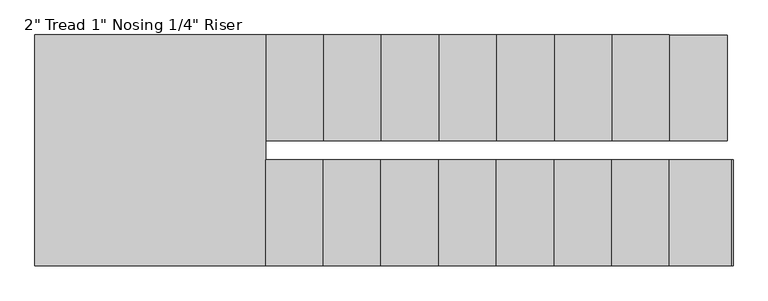
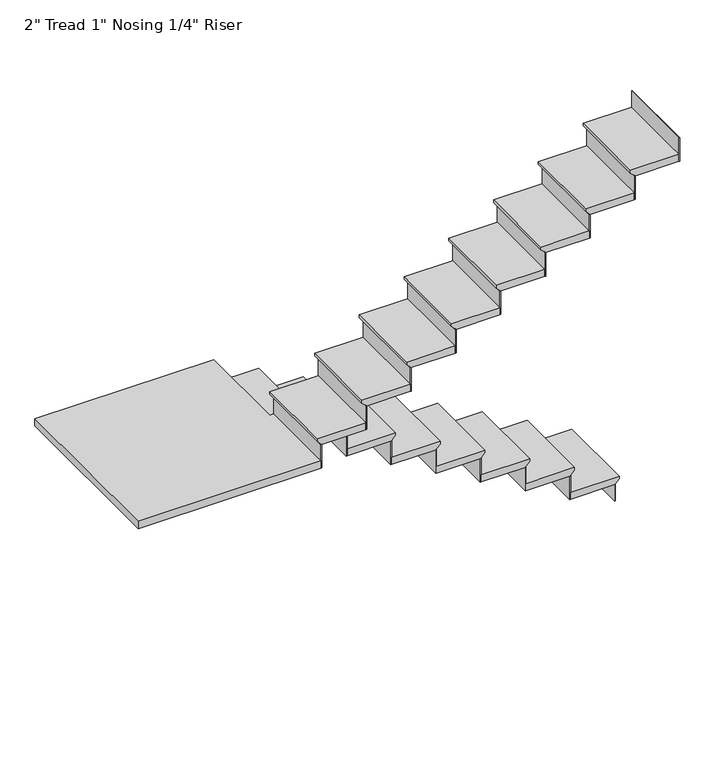
"""IFC4 building model written with IfcOpenShell, lengths in millimetres: stair flight geometry."""

from ifc_helpers import new_model, si_unit, origin, place, context, project, spatial, faceted_brep, source, transform, mapped, element, save


def stair_flight_17867b1e(model_context):
    return source(origin(), model_context, "Body", "Brep", [
        faceted_brep([(-1805.9198569, -5306.3933037, 3350.6833333), (-1805.9198569, -5306.3933037, 3369.7333333), (-1805.9198569, -5865.1933037, 3369.7333333), (-1805.9198569, -5865.1933037, 3350.6833333), (-1831.3198569, -5306.3933037, 3325.2833333), (-1831.3198569, -5865.1933037, 3325.2833333), (-2136.1198569, -5306.3933037, 3369.7333333), (-2136.1198569, -5865.1933037, 3369.7333333), (-1831.3198569, -5865.1933037, 3318.9333333), (-2136.1198569, -5865.1933037, 3318.9333333), (-2136.1198569, -5306.3933037, 3318.9333333), (-1831.3198569, -5306.3933037, 3318.9333333)], [[[0, 1, 2, 3]], [[4, 0, 3, 5]], [[2, 1, 6, 7]], [[8, 9, 10, 11]], [[2, 7, 9, 8, 5, 3]], [[8, 11, 4, 5]], [[6, 1, 0, 4, 11, 10]], [[7, 6, 10, 9]]]),
        faceted_brep([(-1831.3198569, -5306.3933037, 3318.9333333), (-1831.3198569, -5306.3933037, 3200.4), (-1837.6698569, -5306.3933037, 3200.4), (-1837.6698569, -5306.3933037, 3318.9333333), (-1831.3198569, -5865.1933037, 3318.9333333), (-1837.6698569, -5865.1933037, 3318.9333333), (-1837.6698569, -5865.1933037, 3200.4), (-1831.3198569, -5865.1933037, 3200.4)], [[[0, 1, 2, 3]], [[4, 5, 6, 7]], [[1, 0, 4, 7]], [[2, 1, 7, 6]], [[3, 2, 6, 5]], [[0, 3, 5, 4]]]),
        faceted_brep([(-2136.1198569, -5306.3933037, 3488.2666667), (-2136.1198569, -5306.3933037, 3318.9333333), (-2142.4698569, -5306.3933037, 3318.9333333), (-2142.4698569, -5306.3933037, 3488.2666667), (-2136.1198569, -5865.1933037, 3488.2666667), (-2142.4698569, -5865.1933037, 3488.2666667), (-2142.4698569, -5865.1933037, 3318.9333333), (-2136.1198569, -5865.1933037, 3318.9333333)], [[[0, 1, 2, 3]], [[4, 5, 6, 7]], [[1, 0, 4, 7]], [[2, 1, 7, 6]], [[3, 2, 6, 5]], [[0, 3, 5, 4]]]),
        faceted_brep([(-2110.7198569, -5865.1933037, 3539.0666667), (-2110.7198569, -5306.3933037, 3539.0666667), (-2440.9198569, -5306.3933037, 3539.0666667), (-2440.9198569, -5865.1933037, 3539.0666667), (-2136.1198569, -5865.1933037, 3488.2666667), (-2440.9198569, -5865.1933037, 3488.2666667), (-2440.9198569, -5306.3933037, 3488.2666667), (-2136.1198569, -5306.3933037, 3488.2666667), (-2136.1198569, -5865.1933037, 3494.6166667), (-2110.7198569, -5865.1933037, 3520.0166667), (-2136.1198569, -5306.3933037, 3494.6166667), (-2110.7198569, -5306.3933037, 3520.0166667)], [[[0, 1, 2, 3]], [[4, 5, 6, 7]], [[0, 3, 5, 4, 8, 9]], [[4, 7, 10, 8]], [[2, 1, 11, 10, 7, 6]], [[3, 2, 6, 5]], [[11, 1, 0, 9]], [[10, 11, 9, 8]]]),
        faceted_brep([(-2440.9198569, -5306.3933037, 3657.6), (-2440.9198569, -5306.3933037, 3488.2666667), (-2447.2698569, -5306.3933037, 3488.2666667), (-2447.2698569, -5306.3933037, 3657.6), (-2440.9198569, -5865.1933037, 3657.6), (-2447.2698569, -5865.1933037, 3657.6), (-2447.2698569, -5865.1933037, 3488.2666667), (-2440.9198569, -5865.1933037, 3488.2666667)], [[[0, 1, 2, 3]], [[4, 5, 6, 7]], [[1, 0, 4, 7]], [[2, 1, 7, 6]], [[3, 2, 6, 5]], [[0, 3, 5, 4]]]),
        faceted_brep([(-2415.5198569, -5865.1933037, 3708.4), (-2415.5198569, -5306.3933037, 3708.4), (-2745.7198569, -5306.3933037, 3708.4), (-2745.7198569, -5865.1933037, 3708.4), (-2440.9198569, -5865.1933037, 3657.6), (-2745.7198569, -5865.1933037, 3657.6), (-2745.7198569, -5306.3933037, 3657.6), (-2440.9198569, -5306.3933037, 3657.6), (-2440.9198569, -5865.1933037, 3663.95), (-2415.5198569, -5865.1933037, 3689.35), (-2440.9198569, -5306.3933037, 3663.95), (-2415.5198569, -5306.3933037, 3689.35)], [[[0, 1, 2, 3]], [[4, 5, 6, 7]], [[0, 3, 5, 4, 8, 9]], [[4, 7, 10, 8]], [[2, 1, 11, 10, 7, 6]], [[3, 2, 6, 5]], [[11, 1, 0, 9]], [[10, 11, 9, 8]]]),
        faceted_brep([(-2745.7198569, -5306.3933037, 3826.9333333), (-2745.7198569, -5306.3933037, 3657.6), (-2752.0698569, -5306.3933037, 3657.6), (-2752.0698569, -5306.3933037, 3826.9333333), (-2745.7198569, -5865.1933037, 3826.9333333), (-2752.0698569, -5865.1933037, 3826.9333333), (-2752.0698569, -5865.1933037, 3657.6), (-2745.7198569, -5865.1933037, 3657.6)], [[[0, 1, 2, 3]], [[4, 5, 6, 7]], [[1, 0, 4, 7]], [[2, 1, 7, 6]], [[3, 2, 6, 5]], [[0, 3, 5, 4]]]),
        faceted_brep([(-2720.3198569, -5865.1933037, 3877.7333333), (-2720.3198569, -5306.3933037, 3877.7333333), (-3050.5198569, -5306.3933037, 3877.7333333), (-3050.5198569, -5865.1933037, 3877.7333333), (-2745.7198569, -5865.1933037, 3826.9333333), (-3050.5198569, -5865.1933037, 3826.9333333), (-3050.5198569, -5306.3933037, 3826.9333333), (-2745.7198569, -5306.3933037, 3826.9333333), (-2745.7198569, -5865.1933037, 3833.2833333), (-2720.3198569, -5865.1933037, 3858.6833333), (-2745.7198569, -5306.3933037, 3833.2833333), (-2720.3198569, -5306.3933037, 3858.6833333)], [[[0, 1, 2, 3]], [[4, 5, 6, 7]], [[0, 3, 5, 4, 8, 9]], [[4, 7, 10, 8]], [[2, 1, 11, 10, 7, 6]], [[3, 2, 6, 5]], [[11, 1, 0, 9]], [[10, 11, 9, 8]]]),
        faceted_brep([(-3050.5198569, -5306.3933037, 3996.2666667), (-3050.5198569, -5306.3933037, 3826.9333333), (-3056.8698569, -5306.3933037, 3826.9333333), (-3056.8698569, -5306.3933037, 3996.2666667), (-3050.5198569, -5865.1933037, 3996.2666667), (-3056.8698569, -5865.1933037, 3996.2666667), (-3056.8698569, -5865.1933037, 3826.9333333), (-3050.5198569, -5865.1933037, 3826.9333333)], [[[0, 1, 2, 3]], [[4, 5, 6, 7]], [[1, 0, 4, 7]], [[2, 1, 7, 6]], [[3, 2, 6, 5]], [[0, 3, 5, 4]]]),
        faceted_brep([(-3025.1198569, -5865.1933037, 4047.0666667), (-3025.1198569, -5306.3933037, 4047.0666667), (-3355.3198569, -5306.3933037, 4047.0666667), (-3355.3198569, -5865.1933037, 4047.0666667), (-3050.5198569, -5865.1933037, 3996.2666667), (-3355.3198569, -5865.1933037, 3996.2666667), (-3355.3198569, -5306.3933037, 3996.2666667), (-3050.5198569, -5306.3933037, 3996.2666667), (-3050.5198569, -5865.1933037, 4002.6166667), (-3025.1198569, -5865.1933037, 4028.0166667), (-3050.5198569, -5306.3933037, 4002.6166667), (-3025.1198569, -5306.3933037, 4028.0166667)], [[[0, 1, 2, 3]], [[4, 5, 6, 7]], [[0, 3, 5, 4, 8, 9]], [[4, 7, 10, 8]], [[2, 1, 11, 10, 7, 6]], [[3, 2, 6, 5]], [[11, 1, 0, 9]], [[10, 11, 9, 8]]]),
        faceted_brep([(-3355.3198569, -5306.3933037, 4165.6), (-3355.3198569, -5306.3933037, 3996.2666667), (-3361.6698569, -5306.3933037, 3996.2666667), (-3361.6698569, -5306.3933037, 4165.6), (-3355.3198569, -5865.1933037, 4165.6), (-3361.6698569, -5865.1933037, 4165.6), (-3361.6698569, -5865.1933037, 3996.2666667), (-3355.3198569, -5865.1933037, 3996.2666667)], [[[0, 1, 2, 3]], [[4, 5, 6, 7]], [[1, 0, 4, 7]], [[2, 1, 7, 6]], [[3, 2, 6, 5]], [[0, 3, 5, 4]]]),
        faceted_brep([(-3329.9198569, -5865.1933037, 4216.4), (-3329.9198569, -5306.3933037, 4216.4), (-3660.1198569, -5306.3933037, 4216.4), (-3660.1198569, -5865.1933037, 4216.4), (-3355.3198569, -5865.1933037, 4165.6), (-3660.1198569, -5865.1933037, 4165.6), (-3660.1198569, -5306.3933037, 4165.6), (-3355.3198569, -5306.3933037, 4165.6), (-3355.3198569, -5865.1933037, 4171.95), (-3329.9198569, -5865.1933037, 4197.35), (-3355.3198569, -5306.3933037, 4171.95), (-3329.9198569, -5306.3933037, 4197.35)], [[[0, 1, 2, 3]], [[4, 5, 6, 7]], [[0, 3, 5, 4, 8, 9]], [[4, 7, 10, 8]], [[2, 1, 11, 10, 7, 6]], [[3, 2, 6, 5]], [[11, 1, 0, 9]], [[10, 11, 9, 8]]]),
        faceted_brep([(-3660.1198569, -5306.3933037, 4334.9333333), (-3660.1198569, -5306.3933037, 4165.6), (-3666.4698569, -5306.3933037, 4165.6), (-3666.4698569, -5306.3933037, 4334.9333333), (-3660.1198569, -5865.1933037, 4334.9333333), (-3666.4698569, -5865.1933037, 4334.9333333), (-3666.4698569, -5865.1933037, 4165.6), (-3660.1198569, -5865.1933037, 4165.6)], [[[0, 1, 2, 3]], [[4, 5, 6, 7]], [[1, 0, 4, 7]], [[2, 1, 7, 6]], [[3, 2, 6, 5]], [[0, 3, 5, 4]]]),
        faceted_brep([(-3634.7198569, -5865.1933037, 4385.7333333), (-3634.7198569, -5306.3933037, 4385.7333333), (-3964.9198569, -5306.3933037, 4385.7333333), (-3964.9198569, -5865.1933037, 4385.7333333), (-3660.1198569, -5865.1933037, 4334.9333333), (-3964.9198569, -5865.1933037, 4334.9333333), (-3964.9198569, -5306.3933037, 4334.9333333), (-3660.1198569, -5306.3933037, 4334.9333333), (-3660.1198569, -5865.1933037, 4341.2833333), (-3634.7198569, -5865.1933037, 4366.6833333), (-3660.1198569, -5306.3933037, 4341.2833333), (-3634.7198569, -5306.3933037, 4366.6833333)], [[[0, 1, 2, 3]], [[4, 5, 6, 7]], [[0, 3, 5, 4, 8, 9]], [[4, 7, 10, 8]], [[2, 1, 11, 10, 7, 6]], [[3, 2, 6, 5]], [[11, 1, 0, 9]], [[10, 11, 9, 8]]]),
        faceted_brep([(-3964.9198569, -5306.3933037, 4504.2666667), (-3964.9198569, -5306.3933037, 4334.9333333), (-3971.2698569, -5306.3933037, 4334.9333333), (-3971.2698569, -5306.3933037, 4504.2666667), (-3964.9198569, -5865.1933037, 4504.2666667), (-3971.2698569, -5865.1933037, 4504.2666667), (-3971.2698569, -5865.1933037, 4334.9333333), (-3964.9198569, -5865.1933037, 4334.9333333)], [[[0, 1, 2, 3]], [[4, 5, 6, 7]], [[1, 0, 4, 7]], [[2, 1, 7, 6]], [[3, 2, 6, 5]], [[0, 3, 5, 4]]]),
        faceted_brep([(-3939.5198569, -5865.1933037, 4555.0666667), (-3939.5198569, -5306.3933037, 4555.0666667), (-4269.7198569, -5306.3933037, 4555.0666667), (-4269.7198569, -5865.1933037, 4555.0666667), (-3964.9198569, -5865.1933037, 4504.2666667), (-4269.7198569, -5865.1933037, 4504.2666667), (-4269.7198569, -5306.3933037, 4504.2666667), (-3964.9198569, -5306.3933037, 4504.2666667), (-3964.9198569, -5865.1933037, 4510.6166667), (-3939.5198569, -5865.1933037, 4536.0166667), (-3964.9198569, -5306.3933037, 4510.6166667), (-3939.5198569, -5306.3933037, 4536.0166667)], [[[0, 1, 2, 3]], [[4, 5, 6, 7]], [[0, 3, 5, 4, 8, 9]], [[4, 7, 10, 8]], [[2, 1, 11, 10, 7, 6]], [[3, 2, 6, 5]], [[11, 1, 0, 9]], [[10, 11, 9, 8]]]),
        faceted_brep([(-4269.7198569, -5306.3933037, 4673.6), (-4269.7198569, -5306.3933037, 4504.2666667), (-4276.0698569, -5306.3933037, 4504.2666667), (-4276.0698569, -5306.3933037, 4673.6), (-4269.7198569, -5865.1933037, 4673.6), (-4276.0698569, -5865.1933037, 4673.6), (-4276.0698569, -5865.1933037, 4504.2666667), (-4269.7198569, -5865.1933037, 4504.2666667)], [[[0, 1, 2, 3]], [[4, 5, 6, 7]], [[1, 0, 4, 7]], [[2, 1, 7, 6]], [[3, 2, 6, 5]], [[0, 3, 5, 4]]]),
        faceted_brep([(-4218.9198569, -5966.7933037, 4724.4), (-4244.3198569, -5966.7933037, 4724.4), (-4244.3198569, -5306.3933037, 4724.4), (-5463.5198569, -5306.3933037, 4724.4), (-5463.5198569, -6525.5933037, 4724.4), (-4218.9198569, -6525.5933037, 4724.4), (-4244.3198569, -5966.7933037, 4673.6), (-4218.9198569, -5966.7933037, 4673.6), (-4218.9198569, -6525.5933037, 4673.6), (-5463.5198569, -6525.5933037, 4673.6), (-5463.5198569, -5306.3933037, 4673.6), (-4269.7198569, -5306.3933037, 4673.6), (-4269.7198569, -5865.1933037, 4673.6), (-4244.3198569, -5865.1933037, 4673.6), (-4244.3198569, -5865.1933037, 4705.35), (-4244.3198569, -5306.3933037, 4705.35), (-4269.7198569, -5865.1933037, 4679.95), (-4269.7198569, -5306.3933037, 4679.95)], [[[0, 1, 2, 3, 4, 5]], [[6, 7, 8, 9, 10, 11, 12, 13]], [[1, 0, 7, 6]], [[2, 1, 6, 13, 14, 15]], [[13, 12, 16, 14]], [[12, 11, 17, 16]], [[3, 2, 15, 17, 11, 10]], [[4, 3, 10, 9]], [[5, 4, 9, 8]], [[0, 5, 8, 7]], [[17, 15, 14, 16]]]),
        faceted_brep([(-4218.9198569, -6525.5933037, 4842.9333333), (-4218.9198569, -6525.5933037, 4673.6), (-4212.5698569, -6525.5933037, 4673.6), (-4212.5698569, -6525.5933037, 4842.9333333), (-4218.9198569, -5966.7933037, 4842.9333333), (-4212.5698569, -5966.7933037, 4842.9333333), (-4212.5698569, -5966.7933037, 4673.6), (-4218.9198569, -5966.7933037, 4673.6)], [[[0, 1, 2, 3]], [[4, 5, 6, 7]], [[1, 0, 4, 7]], [[2, 1, 7, 6]], [[3, 2, 6, 5]], [[0, 3, 5, 4]]]),
        faceted_brep([(-4244.3198569, -5966.7933037, 4893.7333333), (-4244.3198569, -6525.5933037, 4893.7333333), (-3914.1198569, -6525.5933037, 4893.7333333), (-3914.1198569, -5966.7933037, 4893.7333333), (-4218.9198569, -5966.7933037, 4842.9333333), (-3914.1198569, -5966.7933037, 4842.9333333), (-3914.1198569, -6525.5933037, 4842.9333333), (-4218.9198569, -6525.5933037, 4842.9333333), (-4218.9198569, -5966.7933037, 4849.2833333), (-4244.3198569, -5966.7933037, 4874.6833333), (-4218.9198569, -6525.5933037, 4849.2833333), (-4244.3198569, -6525.5933037, 4874.6833333)], [[[0, 1, 2, 3]], [[4, 5, 6, 7]], [[0, 3, 5, 4, 8, 9]], [[4, 7, 10, 8]], [[2, 1, 11, 10, 7, 6]], [[3, 2, 6, 5]], [[11, 1, 0, 9]], [[10, 11, 9, 8]]]),
        faceted_brep([(-3914.1198569, -6525.5933037, 5012.2666667), (-3914.1198569, -6525.5933037, 4842.9333333), (-3907.7698569, -6525.5933037, 4842.9333333), (-3907.7698569, -6525.5933037, 5012.2666667), (-3914.1198569, -5966.7933037, 5012.2666667), (-3907.7698569, -5966.7933037, 5012.2666667), (-3907.7698569, -5966.7933037, 4842.9333333), (-3914.1198569, -5966.7933037, 4842.9333333)], [[[0, 1, 2, 3]], [[4, 5, 6, 7]], [[1, 0, 4, 7]], [[2, 1, 7, 6]], [[3, 2, 6, 5]], [[0, 3, 5, 4]]]),
        faceted_brep([(-3939.5198569, -5966.7933037, 5063.0666667), (-3939.5198569, -6525.5933037, 5063.0666667), (-3609.3198569, -6525.5933037, 5063.0666667), (-3609.3198569, -5966.7933037, 5063.0666667), (-3914.1198569, -5966.7933037, 5012.2666667), (-3609.3198569, -5966.7933037, 5012.2666667), (-3609.3198569, -6525.5933037, 5012.2666667), (-3914.1198569, -6525.5933037, 5012.2666667), (-3914.1198569, -5966.7933037, 5018.6166667), (-3939.5198569, -5966.7933037, 5044.0166667), (-3914.1198569, -6525.5933037, 5018.6166667), (-3939.5198569, -6525.5933037, 5044.0166667)], [[[0, 1, 2, 3]], [[4, 5, 6, 7]], [[0, 3, 5, 4, 8, 9]], [[4, 7, 10, 8]], [[2, 1, 11, 10, 7, 6]], [[3, 2, 6, 5]], [[11, 1, 0, 9]], [[10, 11, 9, 8]]]),
        faceted_brep([(-3609.3198569, -6525.5933037, 5181.6), (-3609.3198569, -6525.5933037, 5012.2666667), (-3602.9698569, -6525.5933037, 5012.2666667), (-3602.9698569, -6525.5933037, 5181.6), (-3609.3198569, -5966.7933037, 5181.6), (-3602.9698569, -5966.7933037, 5181.6), (-3602.9698569, -5966.7933037, 5012.2666667), (-3609.3198569, -5966.7933037, 5012.2666667)], [[[0, 1, 2, 3]], [[4, 5, 6, 7]], [[1, 0, 4, 7]], [[2, 1, 7, 6]], [[3, 2, 6, 5]], [[0, 3, 5, 4]]]),
        faceted_brep([(-3634.7198569, -5966.7933037, 5232.4), (-3634.7198569, -6525.5933037, 5232.4), (-3304.5198569, -6525.5933037, 5232.4), (-3304.5198569, -5966.7933037, 5232.4), (-3609.3198569, -5966.7933037, 5181.6), (-3304.5198569, -5966.7933037, 5181.6), (-3304.5198569, -6525.5933037, 5181.6), (-3609.3198569, -6525.5933037, 5181.6), (-3609.3198569, -5966.7933037, 5187.95), (-3634.7198569, -5966.7933037, 5213.35), (-3609.3198569, -6525.5933037, 5187.95), (-3634.7198569, -6525.5933037, 5213.35)], [[[0, 1, 2, 3]], [[4, 5, 6, 7]], [[0, 3, 5, 4, 8, 9]], [[4, 7, 10, 8]], [[2, 1, 11, 10, 7, 6]], [[3, 2, 6, 5]], [[11, 1, 0, 9]], [[10, 11, 9, 8]]]),
        faceted_brep([(-3304.5198569, -6525.5933037, 5350.9333333), (-3304.5198569, -6525.5933037, 5181.6), (-3298.1698569, -6525.5933037, 5181.6), (-3298.1698569, -6525.5933037, 5350.9333333), (-3304.5198569, -5966.7933037, 5350.9333333), (-3298.1698569, -5966.7933037, 5350.9333333), (-3298.1698569, -5966.7933037, 5181.6), (-3304.5198569, -5966.7933037, 5181.6)], [[[0, 1, 2, 3]], [[4, 5, 6, 7]], [[1, 0, 4, 7]], [[2, 1, 7, 6]], [[3, 2, 6, 5]], [[0, 3, 5, 4]]]),
        faceted_brep([(-3329.9198569, -5966.7933037, 5401.7333333), (-3329.9198569, -6525.5933037, 5401.7333333), (-2999.7198569, -6525.5933037, 5401.7333333), (-2999.7198569, -5966.7933037, 5401.7333333), (-3304.5198569, -5966.7933037, 5350.9333333), (-2999.7198569, -5966.7933037, 5350.9333333), (-2999.7198569, -6525.5933037, 5350.9333333), (-3304.5198569, -6525.5933037, 5350.9333333), (-3304.5198569, -5966.7933037, 5357.2833333), (-3329.9198569, -5966.7933037, 5382.6833333), (-3304.5198569, -6525.5933037, 5357.2833333), (-3329.9198569, -6525.5933037, 5382.6833333)], [[[0, 1, 2, 3]], [[4, 5, 6, 7]], [[0, 3, 5, 4, 8, 9]], [[4, 7, 10, 8]], [[2, 1, 11, 10, 7, 6]], [[3, 2, 6, 5]], [[11, 1, 0, 9]], [[10, 11, 9, 8]]]),
        faceted_brep([(-2999.7198569, -6525.5933037, 5520.2666667), (-2999.7198569, -6525.5933037, 5350.9333333), (-2993.3698569, -6525.5933037, 5350.9333333), (-2993.3698569, -6525.5933037, 5520.2666667), (-2999.7198569, -5966.7933037, 5520.2666667), (-2993.3698569, -5966.7933037, 5520.2666667), (-2993.3698569, -5966.7933037, 5350.9333333), (-2999.7198569, -5966.7933037, 5350.9333333)], [[[0, 1, 2, 3]], [[4, 5, 6, 7]], [[1, 0, 4, 7]], [[2, 1, 7, 6]], [[3, 2, 6, 5]], [[0, 3, 5, 4]]]),
        faceted_brep([(-3025.1198569, -5966.7933037, 5571.0666667), (-3025.1198569, -6525.5933037, 5571.0666667), (-2694.9198569, -6525.5933037, 5571.0666667), (-2694.9198569, -5966.7933037, 5571.0666667), (-2999.7198569, -5966.7933037, 5520.2666667), (-2694.9198569, -5966.7933037, 5520.2666667), (-2694.9198569, -6525.5933037, 5520.2666667), (-2999.7198569, -6525.5933037, 5520.2666667), (-2999.7198569, -5966.7933037, 5526.6166667), (-3025.1198569, -5966.7933037, 5552.0166667), (-2999.7198569, -6525.5933037, 5526.6166667), (-3025.1198569, -6525.5933037, 5552.0166667)], [[[0, 1, 2, 3]], [[4, 5, 6, 7]], [[0, 3, 5, 4, 8, 9]], [[4, 7, 10, 8]], [[2, 1, 11, 10, 7, 6]], [[3, 2, 6, 5]], [[11, 1, 0, 9]], [[10, 11, 9, 8]]]),
        faceted_brep([(-2694.9198569, -6525.5933037, 5689.6), (-2694.9198569, -6525.5933037, 5520.2666667), (-2688.5698569, -6525.5933037, 5520.2666667), (-2688.5698569, -6525.5933037, 5689.6), (-2694.9198569, -5966.7933037, 5689.6), (-2688.5698569, -5966.7933037, 5689.6), (-2688.5698569, -5966.7933037, 5520.2666667), (-2694.9198569, -5966.7933037, 5520.2666667)], [[[0, 1, 2, 3]], [[4, 5, 6, 7]], [[1, 0, 4, 7]], [[2, 1, 7, 6]], [[3, 2, 6, 5]], [[0, 3, 5, 4]]]),
        faceted_brep([(-2720.3198569, -5966.7933037, 5740.4), (-2720.3198569, -6525.5933037, 5740.4), (-2390.1198569, -6525.5933037, 5740.4), (-2390.1198569, -5966.7933037, 5740.4), (-2694.9198569, -5966.7933037, 5689.6), (-2390.1198569, -5966.7933037, 5689.6), (-2390.1198569, -6525.5933037, 5689.6), (-2694.9198569, -6525.5933037, 5689.6), (-2694.9198569, -5966.7933037, 5695.95), (-2720.3198569, -5966.7933037, 5721.35), (-2694.9198569, -6525.5933037, 5695.95), (-2720.3198569, -6525.5933037, 5721.35)], [[[0, 1, 2, 3]], [[4, 5, 6, 7]], [[0, 3, 5, 4, 8, 9]], [[4, 7, 10, 8]], [[2, 1, 11, 10, 7, 6]], [[3, 2, 6, 5]], [[11, 1, 0, 9]], [[10, 11, 9, 8]]]),
        faceted_brep([(-2390.1198569, -6525.5933037, 5858.9333333), (-2390.1198569, -6525.5933037, 5689.6), (-2383.7698569, -6525.5933037, 5689.6), (-2383.7698569, -6525.5933037, 5858.9333333), (-2390.1198569, -5966.7933037, 5858.9333333), (-2383.7698569, -5966.7933037, 5858.9333333), (-2383.7698569, -5966.7933037, 5689.6), (-2390.1198569, -5966.7933037, 5689.6)], [[[0, 1, 2, 3]], [[4, 5, 6, 7]], [[1, 0, 4, 7]], [[2, 1, 7, 6]], [[3, 2, 6, 5]], [[0, 3, 5, 4]]]),
        faceted_brep([(-2415.5198569, -5966.7933037, 5909.7333333), (-2415.5198569, -6525.5933037, 5909.7333333), (-2085.3198569, -6525.5933037, 5909.7333333), (-2085.3198569, -5966.7933037, 5909.7333333), (-2390.1198569, -5966.7933037, 5858.9333333), (-2085.3198569, -5966.7933037, 5858.9333333), (-2085.3198569, -6525.5933037, 5858.9333333), (-2390.1198569, -6525.5933037, 5858.9333333), (-2390.1198569, -5966.7933037, 5865.2833333), (-2415.5198569, -5966.7933037, 5890.6833333), (-2390.1198569, -6525.5933037, 5865.2833333), (-2415.5198569, -6525.5933037, 5890.6833333)], [[[0, 1, 2, 3]], [[4, 5, 6, 7]], [[0, 3, 5, 4, 8, 9]], [[4, 7, 10, 8]], [[2, 1, 11, 10, 7, 6]], [[3, 2, 6, 5]], [[11, 1, 0, 9]], [[10, 11, 9, 8]]]),
        faceted_brep([(-2085.3198569, -6525.5933037, 6028.2666667), (-2085.3198569, -6525.5933037, 5858.9333333), (-2078.9698569, -6525.5933037, 5858.9333333), (-2078.9698569, -6525.5933037, 6028.2666667), (-2085.3198569, -5966.7933037, 6028.2666667), (-2078.9698569, -5966.7933037, 6028.2666667), (-2078.9698569, -5966.7933037, 5858.9333333), (-2085.3198569, -5966.7933037, 5858.9333333)], [[[0, 1, 2, 3]], [[4, 5, 6, 7]], [[1, 0, 4, 7]], [[2, 1, 7, 6]], [[3, 2, 6, 5]], [[0, 3, 5, 4]]]),
        faceted_brep([(-1780.5198569, -6525.5933037, 6197.6), (-1780.5198569, -6525.5933037, 6028.2666667), (-1774.1698569, -6525.5933037, 6028.2666667), (-1774.1698569, -6525.5933037, 6197.6), (-1780.5198569, -5966.7933037, 6197.6), (-1774.1698569, -5966.7933037, 6197.6), (-1774.1698569, -5966.7933037, 6028.2666667), (-1780.5198569, -5966.7933037, 6028.2666667)], [[[0, 1, 2, 3]], [[4, 5, 6, 7]], [[1, 0, 4, 7]], [[2, 1, 7, 6]], [[3, 2, 6, 5]], [[0, 3, 5, 4]]]),
        faceted_brep([(-2110.7198569, -5966.7933037, 6079.0666667), (-2110.7198569, -6525.5933037, 6079.0666667), (-1780.5198569, -6525.5933037, 6079.0666667), (-1780.5198569, -5966.7933037, 6079.0666667), (-2085.3198569, -5966.7933037, 6028.2666667), (-1780.5198569, -5966.7933037, 6028.2666667), (-1780.5198569, -6525.5933037, 6028.2666667), (-2085.3198569, -6525.5933037, 6028.2666667), (-2085.3198569, -5966.7933037, 6034.6166667), (-2110.7198569, -5966.7933037, 6060.0166667), (-2085.3198569, -6525.5933037, 6034.6166667), (-2110.7198569, -6525.5933037, 6060.0166667)], [[[0, 1, 2, 3]], [[4, 5, 6, 7]], [[0, 3, 5, 4, 8, 9]], [[4, 7, 10, 8]], [[2, 1, 11, 10, 7, 6]], [[3, 2, 6, 5]], [[11, 1, 0, 9]], [[10, 11, 9, 8]]]),
    ])


if __name__ == "__main__":
    model = new_model("IFC4")
    model_context = context("Model", 3, world=origin())
    ifc_project = project(units=[si_unit("LENGTHUNIT", "METRE", prefix="MILLI")], contexts=[model_context])
    site = spatial("IfcSite", under=ifc_project)
    building = spatial("IfcBuilding", under=site)
    placement = place(None, origin())
    stair_flight_shape = stair_flight_17867b1e(model_context)
    element("IfcStairFlight", 1, ObjectType="2\" Tread 1\" Nosing 1/4\" Riser", at=placement, inside=building, context=model_context, shape_type="MappedRepresentation", body=[
        mapped(stair_flight_shape, transform((0.0, 0.0, 0.0), x_axis=(1.0, 0.0, 0.0), y_axis=(0.0, 1.0, 0.0), z_axis=(0.0, 0.0, 1.0))),
    ])
    save(model, "model.ifc")
